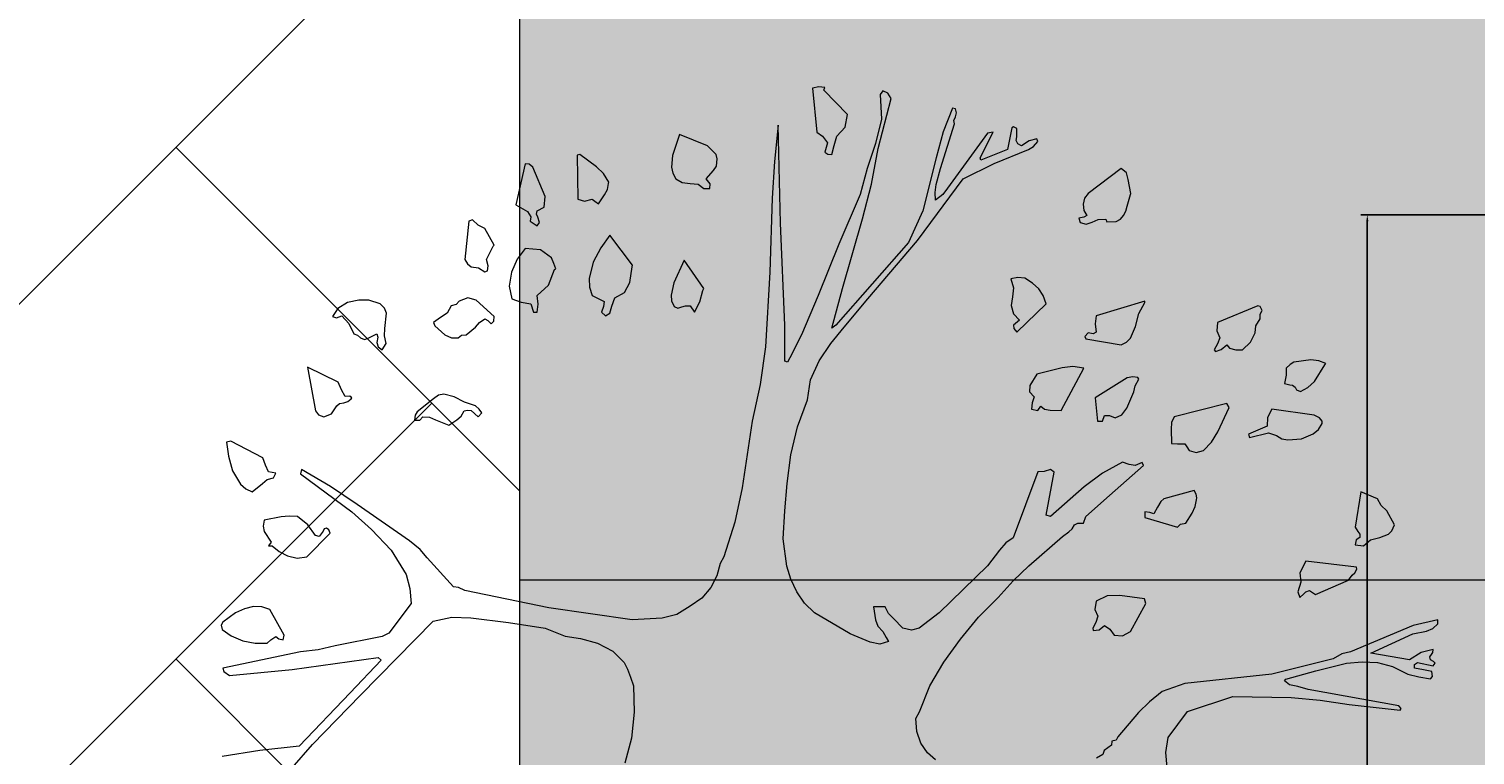
# Model space of a CAD drawing. Units: inches. Extents: x 84 to 1044, y -280 to 906.
# Tile 10 of 105: x 441 to 482, y -46 to -25. Entities that reach past the tile are written whole.
import ezdxf

# ---------------------------------------------------------------- set-up
doc = ezdxf.new("R2010")
doc.units = ezdxf.units.IN
for name, color, linetype, lineweight in [('A-ANNO-DIMS', 2, 'Continuous', 18), ('L-HRDS', 32, 'Continuous', 18), ('L-PLNT', 114, 'Continuous', 15)]:
    doc.layers.add(name, color=color, linetype=linetype, lineweight=lineweight)
for name, color, linetype, lineweight, true_color in [('L-HRDS-PATT', 23, 'Continuous', 9, 0xc2877b), ('L-PLNT-PATT', 9, 'Continuous', 9, 0xafd9aa), ('L-PRKG-PATT', 35, 'Continuous', 9, 0x947764)]:
    doc.layers.add(name, color=color, linetype=linetype, lineweight=lineweight, true_color=true_color)
doc.styles.get("Standard").update_dxf_attribs({"font": 'arial.ttf'})
doc.dimstyles.get("Standard").update_dxf_attribs({"dimtxt": 0.18, "dimasz": 0.18, "dimexe": 0.18, "dimexo": 0.0625, "dimgap": 0.09, "dimtad": 0, "dimtih": 1, "dimtoh": 1, "dimdec": 4, "dimzin": 0, "dimdsep": 46, "dimtxsty": 'Standard', "dimcen": 0.09, "dimadec": 0, "dimazin": 0, "dimtfac": 1, "dimtdec": 4, "dimtofl": 0, "dimtmove": 0, "dimatfit": 3, "dimfxl": 1, "dimtolj": 1, "dimtzin": 0, "dimarcsym": 0})

# ---------------------------------------------------------------- blocks, each defined once
blk = doc.blocks.new('A$C37E508DF')
for p, q in [((0.6329, 1.5111), (0.6367, 1.5175)), ((0.6367, 1.5175), (0.6423, 1.5201)), ((0.6423, 1.5201), (0.6453, 1.5158)), ((0.6453, 1.5158), (0.644, 1.4879)), ((0.6826, 1.493), (0.7096, 1.5209)), ((0.7083, 1.5239), (0.7152, 1.5244)), ((0.7096, 1.5209), (0.7083, 1.5239)), ((0.7152, 1.5244), (0.7225, 1.5231)), ((0.7225, 1.5231), (0.7174, 1.4729)), ((0.5583, 1.4948), (0.5596, 1.4995)), ((0.5596, 1.4995), (0.563, 1.5003)), ((0.563, 1.5003), (0.5737, 1.4733)), ((0.6475, 1.4545), (0.6329, 1.5111)), ((0.5596, 1.4905), (0.5583, 1.4948)), ((0.5613, 1.4862), (0.5596, 1.4905)), ((0.5608, 1.4823), (0.5613, 1.4862)), ((0.644, 1.4879), (0.6505, 1.46)), ((0.6852, 1.4785), (0.6826, 1.493)), ((0.4897, 1.4772), (0.4935, 1.4789)), ((0.4897, 1.4678), (0.4897, 1.4772)), ((0.4905, 1.4635), (0.4897, 1.4678)), ((0.4935, 1.4789), (0.4952, 1.478)), ((0.4952, 1.478), (0.5004, 1.4532)), ((0.5313, 1.4437), (0.5167, 1.4729)), ((0.5167, 1.4729), (0.5231, 1.4716)), ((0.5231, 1.4716), (0.5686, 1.409)), ((0.5767, 1.4317), (0.5608, 1.4823)), ((0.5737, 1.4733), (0.5814, 1.4437)), ((0.6946, 1.4682), (0.6852, 1.4785)), ((0.6976, 1.4579), (0.6946, 1.4682)), ((0.7109, 1.4682), (0.7053, 1.4609)), ((0.7174, 1.4729), (0.7109, 1.4682)), ((0.7589, 1.3691), (0.7615, 1.481)), ((0.7615, 1.481), (0.7658, 1.4395)), ((0.8421, 1.4575), (0.8739, 1.4703)), ((0.8739, 1.4703), (0.882, 1.4463)), ((0.4657, 1.4622), (0.4669, 1.4652)), ((0.4708, 1.4566), (0.4657, 1.4622)), ((0.4669, 1.4652), (0.4755, 1.463)), ((0.4764, 1.4532), (0.4708, 1.4566)), ((0.4755, 1.463), (0.4845, 1.4575)), ((0.5154, 1.4373), (0.4764, 1.4532)), ((0.4845, 1.4575), (0.4884, 1.4596)), ((0.4884, 1.4596), (0.4905, 1.4635)), ((0.5004, 1.4532), (0.5308, 1.4412)), ((0.6552, 1.4137), (0.6475, 1.4545)), ((0.6505, 1.46), (0.6603, 1.4317)), ((0.7002, 1.4476), (0.6976, 1.4579)), ((0.7083, 1.4502), (0.7049, 1.448)), ((0.7053, 1.4609), (0.7083, 1.4502)), ((0.8323, 1.4476), (0.8357, 1.451)), ((0.8357, 1.451), (0.8421, 1.4575)), ((0.551, 1.4197), (0.5154, 1.4373)), ((0.5308, 1.4412), (0.5313, 1.4437)), ((0.5814, 1.4437), (0.5969, 1.3833)), ((0.7049, 1.448), (0.7002, 1.4476)), ((0.7658, 1.4395), (0.7684, 1.3979)), ((0.831, 1.4424), (0.8323, 1.4476)), ((0.8318, 1.4343), (0.831, 1.4424)), ((0.8353, 1.4292), (0.8318, 1.4343)), ((0.8829, 1.433), (0.8816, 1.4262)), ((0.882, 1.4463), (0.8829, 1.433)), ((0.9605, 1.4257), (0.9686, 1.4334)), ((0.9686, 1.4334), (0.9875, 1.4476)), ((0.9875, 1.4476), (0.9905, 1.4467)), ((0.9905, 1.4467), (0.9896, 1.3966)), ((1.0269, 1.3996), (1.0411, 1.433)), ((1.0411, 1.433), (1.045, 1.4365)), ((1.045, 1.4365), (1.0497, 1.4369)), ((1.0497, 1.4369), (1.0604, 1.3901)), ((0.3598, 1.403), (0.3628, 1.4189)), ((0.3628, 1.4189), (0.3649, 1.4266)), ((0.3649, 1.4266), (0.3709, 1.4317)), ((0.3709, 1.4317), (0.4086, 1.403)), ((0.6029, 1.3494), (0.551, 1.4197)), ((0.5814, 1.4133), (0.5767, 1.4317)), ((0.6603, 1.4317), (0.668, 1.4021)), ((0.8434, 1.4197), (0.8353, 1.4292)), ((0.8391, 1.4141), (0.8434, 1.4197)), ((0.8781, 1.4197), (0.8709, 1.4154)), ((0.8816, 1.4262), (0.8781, 1.4197)), ((0.9545, 1.4159), (0.9605, 1.4257)), ((0.3602, 1.4021), (0.3598, 1.403)), ((0.364, 1.3888), (0.3602, 1.4021)), ((0.4086, 1.403), (0.4125, 1.3979)), ((0.5686, 1.409), (0.5741, 1.4021)), ((0.5741, 1.4021), (0.5823, 1.3953)), ((0.5827, 1.4043), (0.5814, 1.4133)), ((0.5823, 1.3953), (0.5827, 1.4043)), ((0.6655, 1.3743), (0.6552, 1.4137)), ((0.668, 1.4021), (0.6925, 1.3455)), ((0.8395, 1.4086), (0.8391, 1.4141)), ((0.846, 1.4086), (0.8395, 1.4086)), ((0.8528, 1.4137), (0.846, 1.4086)), ((0.8619, 1.4146), (0.8528, 1.4137)), ((0.8709, 1.4154), (0.8619, 1.4146)), ((0.9549, 1.4146), (0.9545, 1.4159)), ((0.9558, 1.4077), (0.9549, 1.4146)), ((0.9592, 1.4017), (0.9558, 1.4077)), ((0.966, 1.3914), (0.9592, 1.4017)), ((0.3657, 1.3828), (0.364, 1.3888)), ((0.4134, 1.3837), (0.4099, 1.3781)), ((0.4125, 1.3979), (0.4142, 1.391)), ((0.4142, 1.391), (0.4134, 1.3837)), ((0.7684, 1.3979), (0.771, 1.3134)), ((0.9703, 1.3944), (0.966, 1.3914)), ((0.9733, 1.3966), (0.9703, 1.3944)), ((0.9819, 1.3944), (0.9733, 1.3966)), ((0.9896, 1.3966), (0.9819, 1.3944)), ((1.0282, 1.3876), (1.0269, 1.3996)), ((1.0359, 1.3833), (1.0282, 1.3876)), ((1.0604, 1.3901), (1.0471, 1.3824)), ((0.3683, 1.3781), (0.3657, 1.3828)), ((0.3718, 1.3738), (0.3683, 1.3781)), ((0.3765, 1.3713), (0.3718, 1.3738)), ((0.3872, 1.3708), (0.3765, 1.3713)), ((0.3885, 1.3738), (0.3872, 1.3708)), ((0.3971, 1.3734), (0.3885, 1.3738)), ((0.4039, 1.3704), (0.3971, 1.3734)), ((0.4108, 1.3683), (0.4039, 1.3704)), ((0.4099, 1.3781), (0.4134, 1.376)), ((0.4176, 1.37), (0.4108, 1.3683)), ((0.4134, 1.376), (0.4189, 1.3751)), ((0.4189, 1.3751), (0.4176, 1.37)), ((0.5969, 1.3833), (0.6132, 1.3472)), ((0.6882, 1.2949), (0.6655, 1.3743)), ((0.7538, 1.2529), (0.7589, 1.3691)), ((1.0334, 1.37), (1.0351, 1.376)), ((1.0359, 1.3661), (1.0334, 1.37)), ((1.0351, 1.376), (1.0368, 1.3794)), ((1.0368, 1.3794), (1.0359, 1.3833)), ((1.0441, 1.3717), (1.0359, 1.3661)), ((1.0471, 1.3824), (1.0432, 1.3764)), ((1.0432, 1.3764), (1.0441, 1.3717)), ((1.1033, 1.367), (1.1097, 1.373)), ((1.1097, 1.373), (1.114, 1.3717)), ((1.114, 1.3717), (1.1183, 1.328)), ((0.9274, 1.3215), (0.9532, 1.3554)), ((0.9532, 1.3554), (0.9635, 1.3413)), ((1.0848, 1.3443), (1.0955, 1.3631)), ((1.0955, 1.3631), (1.1033, 1.367)), ((0.6595, 1.2829), (0.6029, 1.3494)), ((0.6132, 1.3472), (0.6959, 1.2529)), ((0.6925, 1.3455), (0.7161, 1.2868)), ((0.9635, 1.3413), (0.9721, 1.325)), ((1.0197, 1.3297), (1.0321, 1.3387)), ((1.0321, 1.3387), (1.0497, 1.3404)), ((1.0497, 1.3404), (1.0587, 1.3284)), ((1.0861, 1.343), (1.0848, 1.3443)), ((1.0938, 1.328), (1.0861, 1.343)), ((0.846, 1.2949), (0.8687, 1.3271)), ((0.8687, 1.3271), (0.8803, 1.3014)), ((0.9279, 1.3194), (0.9274, 1.3215)), ((0.9305, 1.3018), (0.9279, 1.3194)), ((0.9721, 1.325), (0.9768, 1.3061)), ((1.0149, 1.3172), (1.0171, 1.3232)), ((1.0171, 1.3232), (1.0197, 1.3297)), ((1.0587, 1.3284), (1.0651, 1.3134)), ((1.0917, 1.3207), (1.0938, 1.328)), ((1.0925, 1.3151), (1.0917, 1.3207)), ((1.1028, 1.3185), (1.0955, 1.3138)), ((1.111, 1.3194), (1.1028, 1.3185)), ((1.1153, 1.3228), (1.111, 1.3194)), ((1.1183, 1.328), (1.1153, 1.3228)), ((0.4717, 1.3009), (0.4807, 1.3065)), ((0.4807, 1.3065), (0.4884, 1.3074)), ((0.4884, 1.3074), (0.4965, 1.3057)), ((0.4965, 1.3057), (0.4935, 1.2954)), ((0.771, 1.3134), (0.7761, 1.2285)), ((0.8803, 1.3014), (0.8833, 1.2872)), ((0.9365, 1.2902), (0.9305, 1.3018)), ((0.9768, 1.3061), (0.9763, 1.2962)), ((1.0162, 1.3164), (1.0149, 1.3172)), ((1.0231, 1.2988), (1.0162, 1.3164)), ((1.0651, 1.3134), (1.0677, 1.2975)), ((1.0955, 1.3138), (1.0925, 1.3151)), ((0.4562, 1.2774), (0.4597, 1.2868)), ((0.4597, 1.2868), (0.4648, 1.2945)), ((0.4648, 1.2945), (0.4717, 1.3009)), ((0.4935, 1.2954), (0.4948, 1.2855)), ((0.4948, 1.2855), (0.4961, 1.2756)), ((0.7002, 1.2495), (0.6882, 1.2949)), ((0.7161, 1.2868), (0.7349, 1.2422)), ((0.8473, 1.2924), (0.846, 1.2949)), ((0.8507, 1.2795), (0.8473, 1.2924)), ((0.8833, 1.2872), (0.8829, 1.2808)), ((0.9476, 1.2842), (0.9365, 1.2902)), ((0.9733, 1.2868), (0.9596, 1.2799)), ((0.9763, 1.2962), (0.9733, 1.2868)), ((1.0359, 1.2868), (1.0231, 1.2988)), ((1.0347, 1.2769), (1.0359, 1.2868)), ((1.0677, 1.2975), (1.0647, 1.2829)), ((0.2101, 1.2696), (0.2127, 1.2744)), ((0.2127, 1.2654), (0.2101, 1.2696)), ((0.2127, 1.2744), (0.2152, 1.2752)), ((0.2152, 1.2752), (0.2611, 1.2559)), ((0.3439, 1.2804), (0.3992, 1.2636)), ((0.3439, 1.2787), (0.3439, 1.2804)), ((0.3507, 1.2662), (0.3439, 1.2787)), ((0.4897, 1.2452), (0.4562, 1.2774)), ((0.4961, 1.2756), (0.4935, 1.2658)), ((0.6865, 1.2508), (0.6595, 1.2829)), ((0.8567, 1.2679), (0.8507, 1.2795)), ((0.8619, 1.2752), (0.8567, 1.2679)), ((0.867, 1.2752), (0.8619, 1.2752)), ((0.8713, 1.2739), (0.867, 1.2752)), ((0.8756, 1.2726), (0.8713, 1.2739)), ((0.8799, 1.2744), (0.8756, 1.2726)), ((0.8829, 1.2808), (0.8799, 1.2744)), ((0.951, 1.2748), (0.9476, 1.2842)), ((0.9532, 1.2666), (0.951, 1.2748)), ((0.9596, 1.2799), (0.9605, 1.2744)), ((0.9605, 1.2744), (0.9626, 1.2679)), ((1.0359, 1.2679), (1.0347, 1.2769)), ((1.0432, 1.2774), (1.0402, 1.2679)), ((1.0544, 1.2791), (1.0432, 1.2774)), ((1.0647, 1.2829), (1.0544, 1.2791)), ((1.0848, 1.2628), (1.1054, 1.2817)), ((1.1054, 1.2817), (1.1148, 1.2842)), ((1.1148, 1.2842), (1.1247, 1.2804)), ((1.1247, 1.2804), (1.1281, 1.2765)), ((1.1281, 1.2765), (1.1341, 1.2752)), ((1.1341, 1.2752), (1.1384, 1.2666)), ((1.2075, 1.2666), (1.21, 1.2726)), ((1.21, 1.2726), (1.2147, 1.2774)), ((1.2147, 1.2774), (1.2276, 1.2817)), ((1.2276, 1.2817), (1.2392, 1.2817)), ((1.2392, 1.2817), (1.2521, 1.2787)), ((1.2521, 1.2787), (1.2632, 1.2722)), ((1.2632, 1.2722), (1.2692, 1.2628)), ((0.2127, 1.2602), (0.2127, 1.2654)), ((0.2174, 1.2521), (0.2127, 1.2602)), ((0.2182, 1.2443), (0.2174, 1.2521)), ((0.2611, 1.2559), (0.262, 1.2465)), ((0.3546, 1.2516), (0.3507, 1.2662)), ((0.3992, 1.2636), (0.4005, 1.2546)), ((0.4005, 1.2546), (0.3992, 1.2452)), ((0.4935, 1.2658), (0.4867, 1.2589)), ((0.4867, 1.2589), (0.4935, 1.2529)), ((0.4935, 1.2529), (0.4931, 1.2491)), ((0.6959, 1.2529), (0.7002, 1.2495)), ((0.7538, 1.2122), (0.7538, 1.2529)), ((0.9583, 1.2636), (0.9532, 1.2666)), ((0.9626, 1.2679), (0.9583, 1.2636)), ((1.0402, 1.2679), (1.0359, 1.2679)), ((1.0852, 1.2576), (1.0848, 1.2628)), ((1.0883, 1.2546), (1.0852, 1.2576)), ((1.0921, 1.2585), (1.0883, 1.2546)), ((1.0955, 1.2602), (1.0921, 1.2585)), ((1.1015, 1.2559), (1.0955, 1.2602)), ((1.1063, 1.2508), (1.1015, 1.2559)), ((1.1384, 1.2666), (1.1461, 1.2619)), ((1.1526, 1.2521), (1.141, 1.2422)), ((1.1461, 1.2619), (1.1539, 1.2559)), ((1.1539, 1.2559), (1.1526, 1.2521)), ((1.2096, 1.2491), (1.2075, 1.2666)), ((1.2503, 1.2551), (1.2448, 1.2431)), ((1.2585, 1.2636), (1.2503, 1.2551)), ((1.2645, 1.2615), (1.2585, 1.2636)), ((1.2692, 1.2628), (1.2645, 1.2615)), ((0.2234, 1.2336), (0.2182, 1.2443)), ((0.262, 1.2465), (0.2586, 1.2388)), ((0.2586, 1.2388), (0.2611, 1.2319)), ((0.3602, 1.2383), (0.3546, 1.2516)), ((0.3649, 1.2336), (0.3602, 1.2383)), ((0.4112, 1.2375), (0.3709, 1.2306)), ((0.3992, 1.2452), (0.4026, 1.2431)), ((0.4026, 1.2431), (0.4086, 1.2443)), ((0.4086, 1.2443), (0.4121, 1.2401)), ((0.4121, 1.2401), (0.4112, 1.2375)), ((0.4931, 1.2491), (0.4897, 1.2452)), ((0.7015, 1.2323), (0.6865, 1.2508)), ((0.7349, 1.2422), (0.7482, 1.216)), ((1.117, 1.2422), (1.1063, 1.2508)), ((1.1221, 1.2418), (1.117, 1.2422)), ((1.126, 1.2388), (1.1221, 1.2418)), ((1.1337, 1.2388), (1.126, 1.2388)), ((1.141, 1.2422), (1.1337, 1.2388)), ((1.2079, 1.2323), (1.21, 1.2409)), ((1.21, 1.2409), (1.2096, 1.2491)), ((1.2186, 1.2431), (1.2173, 1.2392)), ((1.2173, 1.2392), (1.2186, 1.2332)), ((1.2285, 1.2383), (1.2186, 1.2431)), ((1.2328, 1.2366), (1.2285, 1.2383)), ((1.2371, 1.2388), (1.2328, 1.2366)), ((1.2405, 1.2418), (1.2371, 1.2388)), ((1.2448, 1.2431), (1.2405, 1.2418)), ((0.2328, 1.2251), (0.2234, 1.2336)), ((0.2401, 1.2251), (0.2328, 1.2251)), ((0.2474, 1.2268), (0.2401, 1.2251)), ((0.2504, 1.2306), (0.2474, 1.2268)), ((0.2568, 1.2255), (0.2504, 1.2306)), ((0.2633, 1.2229), (0.2568, 1.2255)), ((0.2611, 1.2319), (0.265, 1.2251)), ((0.265, 1.2251), (0.2633, 1.2229)), ((0.3709, 1.2306), (0.3649, 1.2336)), ((0.7148, 1.2126), (0.7015, 1.2323)), ((0.7761, 1.2285), (0.7821, 1.1856)), ((1.2126, 1.2251), (1.2079, 1.2323)), ((1.2169, 1.2285), (1.2126, 1.2251)), ((1.2186, 1.2332), (1.2169, 1.2285)), ((0.1376, 1.2092), (0.1458, 1.2126)), ((0.1389, 1.2079), (0.1376, 1.2092)), ((0.1505, 1.189), (0.1389, 1.2079)), ((0.1458, 1.2126), (0.1548, 1.2135)), ((0.1548, 1.2135), (0.1741, 1.2109)), ((0.1741, 1.2109), (0.1784, 1.2083)), ((0.1784, 1.2083), (0.1831, 1.204)), ((0.1831, 1.204), (0.1831, 1.1959)), ((0.4134, 1.204), (0.4258, 1.2058)), ((0.4391, 1.156), (0.4134, 1.204)), ((0.4258, 1.2058), (0.4382, 1.2045)), ((0.4382, 1.2045), (0.4669, 1.1972)), ((0.7246, 1.1908), (0.7148, 1.2126)), ((0.7482, 1.216), (0.7508, 1.2109)), ((0.7508, 1.2109), (0.7538, 1.2122)), ((1.2628, 1.1882), (1.2975, 1.2053)), ((1.2975, 1.2053), (1.2885, 1.1556)), ((0.1582, 1.1822), (0.1505, 1.189)), ((0.1848, 1.1865), (0.1788, 1.1852)), ((0.1831, 1.1959), (0.1848, 1.1865)), ((0.3507, 1.1916), (0.352, 1.1933)), ((0.355, 1.1839), (0.3507, 1.1916)), ((0.352, 1.1933), (0.3576, 1.1942)), ((0.3576, 1.1942), (0.364, 1.1929)), ((0.364, 1.1929), (0.4005, 1.1702)), ((0.4669, 1.1972), (0.4747, 1.1843)), ((0.7281, 1.168), (0.7246, 1.1908)), ((1.2589, 1.1792), (1.2628, 1.1882)), ((0.1668, 1.1775), (0.1582, 1.1822)), ((0.1711, 1.1792), (0.1668, 1.1775)), ((0.1728, 1.1826), (0.1711, 1.1792)), ((0.1758, 1.1847), (0.1728, 1.1826)), ((0.1788, 1.1852), (0.1758, 1.1847)), ((0.3563, 1.177), (0.355, 1.1839)), ((0.3645, 1.1586), (0.3563, 1.177)), ((0.4005, 1.1702), (0.3979, 1.1436)), ((0.4751, 1.177), (0.47, 1.1714)), ((0.47, 1.1714), (0.4721, 1.1646)), ((0.4747, 1.1843), (0.4751, 1.177)), ((0.7821, 1.1856), (0.7911, 1.1436)), ((1.1187, 1.1655), (1.1307, 1.1714)), ((1.1307, 1.1714), (1.1423, 1.1744)), ((1.1423, 1.1744), (1.1483, 1.1732)), ((1.1483, 1.1732), (1.1539, 1.1693)), ((1.2469, 1.1702), (1.2495, 1.1723)), ((1.2478, 1.1693), (1.2469, 1.1702)), ((1.2495, 1.1723), (1.2546, 1.1719)), ((1.2546, 1.1719), (1.2589, 1.1792)), ((0.1509, 1.1504), (0.1994, 1.1573)), ((0.1994, 1.1573), (0.2041, 1.1479)), ((0.2478, 1.1594), (0.2504, 1.1637)), ((0.2607, 1.1316), (0.2478, 1.1594)), ((0.2504, 1.1637), (0.3104, 1.1487)), ((0.37, 1.1509), (0.3645, 1.1586)), ((0.4519, 1.1564), (0.4391, 1.156)), ((0.458, 1.1573), (0.4519, 1.1564)), ((0.4622, 1.1607), (0.458, 1.1573)), ((0.4657, 1.156), (0.4622, 1.1607)), ((0.473, 1.1573), (0.4657, 1.156)), ((0.4721, 1.1646), (0.473, 1.1573)), ((0.7396, 1.1371), (0.7281, 1.168)), ((1.099, 1.153), (1.102, 1.1573)), ((1.1033, 1.1487), (1.099, 1.153)), ((1.102, 1.1573), (1.1063, 1.1612)), ((1.111, 1.156), (1.1033, 1.1487)), ((1.1063, 1.1612), (1.1187, 1.1655)), ((1.1153, 1.1564), (1.111, 1.156)), ((1.1191, 1.1556), (1.1153, 1.1564)), ((1.1226, 1.1492), (1.1191, 1.1556)), ((1.1539, 1.1693), (1.1727, 1.1543)), ((1.1727, 1.1543), (1.1749, 1.1504)), ((1.2516, 1.1659), (1.2478, 1.1693)), ((1.2563, 1.1646), (1.2516, 1.1659)), ((1.2611, 1.1637), (1.2563, 1.1646)), ((1.2641, 1.1612), (1.2611, 1.1637)), ((1.2701, 1.1522), (1.2641, 1.1612)), ((1.2885, 1.1556), (1.2851, 1.1509)), ((0.1419, 1.1436), (0.1449, 1.1474)), ((0.1419, 1.141), (0.1419, 1.1436)), ((0.1462, 1.1342), (0.1419, 1.141)), ((0.1449, 1.1474), (0.1509, 1.1504)), ((0.2041, 1.1479), (0.2045, 1.138)), ((0.2045, 1.138), (0.226, 1.129)), ((0.3104, 1.1487), (0.3134, 1.1423)), ((0.3134, 1.1423), (0.3139, 1.1346)), ((0.3778, 1.1474), (0.37, 1.1509)), ((0.3842, 1.15), (0.3778, 1.1474)), ((0.3898, 1.15), (0.3842, 1.15)), ((0.3923, 1.1436), (0.3898, 1.15)), ((0.3979, 1.1436), (0.3923, 1.1436)), ((0.7469, 1.1054), (0.7396, 1.1371)), ((0.7911, 1.1436), (0.8027, 1.0677)), ((1.1273, 1.1453), (1.1226, 1.1492)), ((1.1367, 1.1393), (1.1273, 1.1453)), ((1.1517, 1.1453), (1.1367, 1.1393)), ((1.1586, 1.1483), (1.1517, 1.1453)), ((1.1663, 1.1487), (1.1586, 1.1483)), ((1.1697, 1.1449), (1.1663, 1.1487)), ((1.1757, 1.1449), (1.1697, 1.1449)), ((1.1749, 1.1504), (1.1757, 1.1449)), ((1.2791, 1.1487), (1.2701, 1.1522)), ((1.2851, 1.1509), (1.2791, 1.1487)), ((0.1522, 1.1294), (0.1462, 1.1342)), ((0.1655, 1.1234), (0.1522, 1.1294)), ((0.181, 1.1226), (0.1655, 1.1234)), ((0.1878, 1.1234), (0.181, 1.1226)), ((0.1938, 1.1273), (0.1878, 1.1234)), ((0.2032, 1.1303), (0.1938, 1.1273)), ((0.2247, 1.1251), (0.2032, 1.1303)), ((0.226, 1.129), (0.2247, 1.1251)), ((0.268, 1.1196), (0.2607, 1.1316)), ((0.3139, 1.1346), (0.3134, 1.1183)), ((1.3485, 1.102), (1.385, 1.1209)), ((1.385, 1.1209), (1.3897, 1.1196)), ((0.277, 1.1101), (0.268, 1.1196)), ((0.2856, 1.108), (0.277, 1.1101)), ((0.2933, 1.1101), (0.2856, 1.108)), ((0.2959, 1.1144), (0.2933, 1.1101)), ((0.2984, 1.1179), (0.2959, 1.1144)), ((0.3066, 1.1179), (0.2984, 1.1179)), ((0.3134, 1.1183), (0.3066, 1.1179)), ((0.7512, 1.0728), (0.7469, 1.1054)), ((1.3875, 1.1037), (1.3828, 1.087)), ((1.3897, 1.1196), (1.3875, 1.1037)), ((0.3456, 1.093), (0.3469, 1.0964)), ((0.3842, 1.0591), (0.3456, 1.093)), ((0.3469, 1.0964), (0.355, 1.093)), ((0.355, 1.093), (0.3619, 1.0943)), ((0.3619, 1.0943), (0.3692, 1.0968)), ((0.3692, 1.0968), (0.3923, 1.0844)), ((0.4472, 1.0857), (0.4515, 1.0887)), ((0.4515, 1.0887), (0.4584, 1.0865)), ((1.2713, 1.0694), (1.3044, 1.0887)), ((1.3044, 1.0887), (1.3057, 1.0835)), ((1.3421, 1.0861), (1.3455, 1.0934)), ((1.3455, 1.0934), (1.3485, 1.102)), ((0.3923, 1.0844), (0.4129, 1.069)), ((0.4562, 1.0364), (0.4472, 1.0857)), ((0.4584, 1.0865), (0.4657, 1.0861)), ((0.4657, 1.0861), (0.4939, 1.0107)), ((0.7538, 1.0415), (0.7512, 1.0728)), ((1.3057, 1.0835), (1.2469, 1.0402)), ((1.3335, 1.0844), (1.3421, 1.0861)), ((1.3361, 1.0793), (1.3335, 1.0844)), ((1.3434, 1.0771), (1.3361, 1.0793)), ((1.349, 1.0728), (1.3434, 1.0771)), ((1.3605, 1.063), (1.349, 1.0728)), ((1.3738, 1.072), (1.3678, 1.0664)), ((1.3828, 1.087), (1.3738, 1.072)), ((0.0746, 1.0475), (0.0789, 1.0552)), ((0.0789, 1.0552), (0.0978, 1.063)), ((0.0978, 1.063), (0.1042, 1.0231)), ((0.2847, 1.0565), (0.2856, 1.0604)), ((0.2851, 1.054), (0.2847, 1.0565)), ((0.2856, 1.0604), (0.2877, 1.0647)), ((0.2877, 1.0647), (0.3224, 1.0552)), ((0.3224, 1.0552), (0.3255, 1.0522)), ((0.4112, 1.0351), (0.3842, 1.0591)), ((0.4129, 1.069), (0.4515, 1.0351)), ((0.8027, 1.0677), (0.8108, 1.0287)), ((1.2409, 1.0488), (1.2713, 1.0694)), ((1.3678, 1.0664), (1.3605, 1.063)), ((0.0596, 1.0257), (0.0682, 1.0415)), ((0.0682, 1.0415), (0.0746, 1.0475)), ((0.2864, 1.0463), (0.2851, 1.054)), ((0.2899, 1.039), (0.2864, 1.0463)), ((0.2972, 1.0274), (0.2899, 1.039)), ((0.3255, 1.0522), (0.3293, 1.0458)), ((0.3293, 1.0458), (0.3336, 1.0381)), ((0.3336, 1.0381), (0.3383, 1.0398)), ((0.3383, 1.0398), (0.3439, 1.0402)), ((0.3439, 1.0402), (0.3439, 1.0338)), ((0.7559, 1.0098), (0.7538, 1.0415)), ((1.1813, 1.0072), (1.2409, 1.0488)), ((1.2469, 1.0402), (1.2246, 1.0201)), ((0.0626, 1.0188), (0.0596, 1.0257)), ((0.1042, 1.0231), (0.1012, 1.018)), ((0.3032, 1.0265), (0.2972, 1.0274)), ((0.3066, 1.0231), (0.3032, 1.0265)), ((0.3439, 1.0338), (0.3066, 1.0231)), ((0.4138, 1.0274), (0.4112, 1.0351)), ((0.4202, 1.0274), (0.4138, 1.0274)), ((0.4241, 1.0257), (0.4202, 1.0274)), ((0.4267, 1.0209), (0.4241, 1.0257)), ((0.4515, 1.0351), (0.4562, 1.0364)), ((0.8108, 1.0287), (0.8233, 0.9892)), ((1.2731, 1.0197), (1.2761, 1.0218)), ((1.2761, 1.0218), (1.2786, 1.0209)), ((1.2885, 1.0136), (1.2971, 1.0257)), ((1.2971, 1.0257), (1.3091, 1.0351)), ((1.3091, 1.0351), (1.3185, 1.0355)), ((1.3185, 1.0355), (1.3275, 1.0347)), ((1.3275, 1.0347), (1.3468, 1.0308)), ((1.3468, 1.0308), (1.3481, 1.0239)), ((1.3481, 1.0239), (1.3468, 1.018)), ((0.0665, 1.0149), (0.0626, 1.0188)), ((0.0763, 1.0111), (0.0665, 1.0149)), ((0.087, 1.0085), (0.0763, 1.0111)), ((0.0948, 1.0016), (0.087, 1.0085)), ((0.1012, 1.018), (0.099, 1.0149)), ((0.099, 1.0149), (0.099, 1.0111)), ((0.099, 1.0111), (0.1033, 1.0085)), ((0.1033, 1.0085), (0.1042, 1.0029)), ((0.4305, 1.0175), (0.4267, 1.0209)), ((0.4378, 1.0124), (0.4305, 1.0175)), ((0.476, 0.9789), (0.4378, 1.0124)), ((0.4939, 1.0107), (0.5021, 1.0051)), ((0.5021, 1.0051), (0.5094, 0.9969)), ((0.7516, 0.9785), (0.7559, 1.0098)), ((1.1693, 0.9974), (1.1813, 1.0072)), ((1.2246, 1.0201), (1.2023, 0.9969)), ((1.2718, 1.0162), (1.2731, 1.0197)), ((1.2984, 0.9892), (1.2718, 1.0162)), ((1.2786, 1.0209), (1.2799, 1.0184)), ((1.2799, 1.0184), (1.2842, 1.0124)), ((1.2842, 1.0124), (1.2885, 1.0136)), ((1.3468, 1.018), (1.3391, 1.0059)), ((1.3391, 1.0059), (1.3421, 1.0016)), ((0.1042, 1.0029), (0.0948, 1.0016)), ((0.5094, 0.9969), (0.5231, 0.9789)), ((0.8233, 0.9892), (0.8275, 0.9815)), ((1.1612, 0.9879), (1.1693, 0.9974)), ((1.2023, 0.9969), (1.1852, 0.9691)), ((1.3095, 0.9875), (1.2984, 0.9892)), ((1.3202, 0.9901), (1.3095, 0.9875)), ((1.3297, 0.9952), (1.3202, 0.9901)), ((1.3378, 1.0016), (1.3297, 0.9952)), ((1.3421, 1.0016), (1.3378, 1.0016)), ((0.1025, 0.9751), (0.1029, 0.9772)), ((0.1046, 0.9708), (0.1025, 0.9751)), ((0.1029, 0.9772), (0.1604, 0.9841)), ((0.1604, 0.9841), (0.1672, 0.9708)), ((0.4939, 0.9618), (0.476, 0.9789)), ((0.5231, 0.9789), (0.578, 0.9253)), ((0.7469, 0.9635), (0.7516, 0.9785)), ((0.8275, 0.9815), (0.8314, 0.9673)), ((1.1311, 0.9549), (1.1612, 0.9879)), ((0.1076, 0.9682), (0.1046, 0.9708)), ((0.1119, 0.9626), (0.1076, 0.9682)), ((0.1496, 0.9463), (0.1119, 0.9626)), ((0.1672, 0.9708), (0.1664, 0.9601)), ((0.1664, 0.9601), (0.1698, 0.9493)), ((0.5111, 0.9429), (0.4939, 0.9618)), ((0.7401, 0.9493), (0.7469, 0.9635)), ((0.8314, 0.9673), (0.8383, 0.954)), ((1.1852, 0.9691), (1.1809, 0.9532)), ((0.1565, 0.9506), (0.1496, 0.9463)), ((0.1604, 0.9493), (0.1565, 0.9506)), ((0.1629, 0.9468), (0.1604, 0.9493)), ((0.1672, 0.9429), (0.1629, 0.9468)), ((0.1698, 0.9493), (0.1672, 0.9429)), ((0.3426, 0.936), (0.3443, 0.9412)), ((0.3443, 0.9412), (0.3722, 0.9451)), ((0.3722, 0.9451), (0.3868, 0.9446)), ((0.3868, 0.9446), (0.3992, 0.9386)), ((0.5334, 0.9202), (0.5111, 0.9429)), ((0.7315, 0.9365), (0.7401, 0.9493)), ((0.8383, 0.954), (0.8486, 0.942)), ((0.8486, 0.942), (0.8619, 0.933)), ((1.0227, 0.9309), (1.1183, 0.9506)), ((1.1183, 0.9506), (1.1256, 0.954)), ((1.1256, 0.954), (1.1311, 0.9549)), ((1.1809, 0.9532), (1.1796, 0.936)), ((0.3602, 0.9039), (0.3426, 0.936)), ((0.4009, 0.9292), (0.3975, 0.9215)), ((0.3992, 0.9386), (0.4009, 0.9292)), ((0.578, 0.9253), (0.6011, 0.9077)), ((0.6303, 0.9189), (0.6359, 0.9245)), ((0.6359, 0.9245), (0.6397, 0.9322)), ((0.6397, 0.9322), (0.653, 0.9322)), ((0.653, 0.9322), (0.6505, 0.9172)), ((0.6796, 0.9013), (0.7203, 0.9253)), ((0.7203, 0.9253), (0.7315, 0.9365)), ((0.8619, 0.933), (0.8769, 0.9236)), ((0.8769, 0.9236), (0.8936, 0.9193)), ((0.9279, 0.9172), (1.0227, 0.9309)), ((1.1796, 0.936), (1.2049, 0.9022)), ((1.3241, 0.9), (1.3404, 0.9292)), ((1.3404, 0.9292), (1.3494, 0.9322)), ((1.3494, 0.9322), (1.3592, 0.9326)), ((1.3592, 0.9326), (1.3695, 0.93)), ((1.3695, 0.93), (1.3794, 0.9253)), ((1.3794, 0.9253), (1.394, 0.9146)), ((0.0103, 0.9129), (0.0103, 0.9172)), ((0.0103, 0.9172), (0.0382, 0.9107)), ((0.0159, 0.9073), (0.0103, 0.9129)), ((0.0232, 0.9043), (0.0159, 0.9073)), ((0.0382, 0.9107), (0.1098, 0.8807)), ((0.3838, 0.9069), (0.379, 0.9)), ((0.3898, 0.9107), (0.3838, 0.9069)), ((0.3958, 0.906), (0.3898, 0.9107)), ((0.4026, 0.9052), (0.3958, 0.906)), ((0.3975, 0.9215), (0.3996, 0.9142)), ((0.3996, 0.9142), (0.4031, 0.9077)), ((0.4031, 0.9077), (0.4026, 0.9052)), ((0.554, 0.8953), (0.5334, 0.9202)), ((0.6011, 0.9077), (0.6097, 0.9056)), ((0.6097, 0.9056), (0.6196, 0.9077)), ((0.6196, 0.9077), (0.6303, 0.9189)), ((0.6479, 0.9103), (0.6423, 0.9039)), ((0.6505, 0.9172), (0.6479, 0.9103)), ((0.8936, 0.9193), (0.9279, 0.9172)), ((1.0269, 0.9077), (1.0042, 0.8987)), ((1.0685, 0.9142), (1.0269, 0.9077)), ((1.1114, 0.9198), (1.0685, 0.9142)), ((1.1333, 0.9202), (1.1114, 0.9198)), ((1.1543, 0.9159), (1.1333, 0.9202)), ((1.2371, 0.8314), (1.1543, 0.9159)), ((1.3948, 0.9065), (1.3846, 0.8992)), ((1.394, 0.9146), (1.3957, 0.9112)), ((1.3957, 0.9112), (1.3948, 0.9065)), ((0.0386, 0.9013), (0.0232, 0.9043)), ((0.0866, 0.8794), (0.0386, 0.9013)), ((0.3692, 0.8992), (0.3602, 0.9039)), ((0.379, 0.9), (0.3692, 0.8992)), ((0.5728, 0.8691), (0.554, 0.8953)), ((0.6384, 0.8974), (0.6359, 0.8927)), ((0.6359, 0.8927), (0.6457, 0.8897)), ((0.6423, 0.9039), (0.6384, 0.8974)), ((0.6457, 0.8897), (0.6569, 0.8919)), ((0.6569, 0.8919), (0.6796, 0.9013)), ((0.9673, 0.8906), (0.9498, 0.8816)), ((0.9866, 0.8962), (0.9673, 0.8906)), ((1.0042, 0.8987), (0.9866, 0.8962)), ((1.2049, 0.9022), (1.2126, 0.8983)), ((1.2126, 0.8983), (1.2662, 0.8876)), ((1.3254, 0.8944), (1.3241, 0.9)), ((1.3301, 0.8957), (1.3254, 0.8944)), ((1.3335, 0.8983), (1.3301, 0.8957)), ((1.3395, 0.8944), (1.3335, 0.8983)), ((1.3434, 0.8906), (1.3395, 0.8944)), ((1.3571, 0.8906), (1.3434, 0.8906)), ((1.3713, 0.8936), (1.3571, 0.8906)), ((1.3846, 0.8992), (1.3713, 0.8936)), ((0.0159, 0.8803), (0.0154, 0.8837)), ((0.0154, 0.8837), (0.0292, 0.8803)), ((0.0176, 0.8777), (0.0159, 0.8803)), ((0.0193, 0.8752), (0.0176, 0.8777)), ((0.0184, 0.8717), (0.0193, 0.8752)), ((0.0292, 0.8803), (0.0424, 0.8717)), ((0.0424, 0.8717), (0.0866, 0.8794)), ((0.1098, 0.8807), (0.1196, 0.8786)), ((0.1196, 0.8786), (0.1295, 0.873)), ((0.1295, 0.873), (0.1994, 0.8554)), ((0.9498, 0.8816), (0.9369, 0.8687)), ((1.2169, 0.8743), (1.2135, 0.8713)), ((1.3151, 0.8606), (1.2169, 0.8743)), ((1.2662, 0.8876), (1.2855, 0.8833)), ((1.2855, 0.8833), (1.3057, 0.8807)), ((1.3057, 0.8807), (1.394, 0.8623)), ((0.0133, 0.8679), (0.015, 0.87)), ((0.0154, 0.8649), (0.0133, 0.8679)), ((0.015, 0.87), (0.0184, 0.8717)), ((0.0334, 0.8687), (0.0154, 0.8649)), ((0.0163, 0.8529), (0.0171, 0.8584)), ((0.0171, 0.8584), (0.0266, 0.8602)), ((0.0266, 0.8602), (0.0369, 0.8623)), ((0.0369, 0.8666), (0.0334, 0.8687)), ((0.0369, 0.8623), (0.0369, 0.8666)), ((0.0617, 0.864), (0.0442, 0.8554)), ((0.0789, 0.8687), (0.0617, 0.864)), ((0.0965, 0.8696), (0.0789, 0.8687)), ((0.1141, 0.8679), (0.0965, 0.8696)), ((0.1492, 0.8593), (0.1141, 0.8679)), ((0.1835, 0.8499), (0.1492, 0.8593)), ((0.5887, 0.8421), (0.5728, 0.8691)), ((0.933, 0.861), (0.9296, 0.852)), ((0.9369, 0.8687), (0.933, 0.861)), ((1.2135, 0.8713), (1.2491, 0.834)), ((1.3863, 0.8541), (1.3151, 0.8606)), ((1.3927, 0.8584), (1.3863, 0.8541)), ((1.394, 0.8623), (1.3927, 0.8584)), ((0.0184, 0.8503), (0.0163, 0.8529)), ((0.0317, 0.8524), (0.0184, 0.8503)), ((0.0442, 0.8554), (0.0317, 0.8524)), ((0.1578, 0.8378), (0.1698, 0.8413)), ((0.1698, 0.8413), (0.1792, 0.8434)), ((0.1792, 0.8434), (0.1848, 0.8477)), ((0.1848, 0.8477), (0.1835, 0.8499)), ((0.1994, 0.8554), (0.2984, 0.8447)), ((0.2984, 0.8447), (0.3242, 0.8357)), ((0.6007, 0.8125), (0.5887, 0.8421)), ((0.9262, 0.8421), (0.9257, 0.8121)), ((0.9296, 0.852), (0.9262, 0.8421)), ((0.0545, 0.8194), (0.1578, 0.8378)), ((0.1441, 0.8258), (0.1111, 0.8207)), ((0.1771, 0.8288), (0.1441, 0.8258)), ((0.2436, 0.8301), (0.1771, 0.8288)), ((0.2954, 0.813), (0.2436, 0.8301)), ((0.3242, 0.8357), (0.3387, 0.8241)), ((0.3387, 0.8241), (0.3512, 0.8117)), ((1.2919, 0.7752), (1.2371, 0.8314)), ((1.2491, 0.834), (1.3069, 0.7735)), ((0.0519, 0.8164), (0.0545, 0.8194)), ((0.0532, 0.8143), (0.0519, 0.8164)), ((0.1111, 0.8207), (0.0532, 0.8143)), ((0.3173, 0.7834), (0.2954, 0.813)), ((0.3512, 0.8117), (0.3748, 0.7842)), ((0.6046, 0.8048), (0.6007, 0.8125)), ((0.9257, 0.8121), (0.9287, 0.7825)), ((0.6037, 0.7903), (0.6046, 0.8048)), ((0.3199, 0.7662), (0.3173, 0.7834)), ((0.3748, 0.7842), (0.3765, 0.7804)), ((0.3765, 0.7804), (0.3816, 0.7791)), ((0.3816, 0.7791), (0.382, 0.7744)), ((0.382, 0.7744), (0.3859, 0.7714)), ((0.5913, 0.7658), (0.599, 0.777)), ((0.599, 0.777), (0.6037, 0.7903)), ((0.9287, 0.7825), (0.936, 0.7542)), ((1.3151, 0.7487), (1.2919, 0.7752)), ((0.3186, 0.7491), (0.3199, 0.7662)), ((0.3859, 0.7714), (0.3902, 0.7684)), ((0.3902, 0.7684), (0.3919, 0.7641)), ((0.3919, 0.7641), (0.3988, 0.7598)), ((0.5823, 0.7577), (0.5913, 0.7658)), ((1.3069, 0.7735), (1.352, 0.7684)), ((1.352, 0.7684), (1.3948, 0.7615))]:
    blk.add_line(p, q)
blk = doc.blocks.new('*D28')
at = {"layer": 'A-ANNO-DIMS', "color": 0, "lineweight": -2, "transparency": 16777216}
for p, q in [((484.443, -30.627), (478.69, -30.627)), ((478.87, -30.807), (478.87, -49.227)), ((478.87, -68.013), (478.87, -49.593)), ((484.443, -68.193), (478.69, -68.193))]:
    blk.add_line(p, q, dxfattribs=at)
at = {"layer": 'A-ANNO-DIMS', "color": 0, "transparency": 16777216}
for points in [[(478.84, -30.807), (478.9, -30.807), (478.87, -30.627)], [(478.84, -68.013), (478.9, -68.013), (478.87, -68.193)]]:
    blk.add_solid(points, dxfattribs=at)
at = {"layer": 'Defpoints', "color": 0, "transparency": 16777216}
for p in [(478.87, -30.627), (484.505, -30.627), (484.505, -68.193)]:
    blk.add_point(p, dxfattribs=at)
at = {"layer": 'A-ANNO-DIMS', "color": 0, "transparency": 16777216, "insert": (478.87, -49.41), "char_height": 0.18, "attachment_point": 5}
blk.add_mtext('\\A1;SHRUB 38 TYP.', dxfattribs=at)

msp = doc.modelspace()

# ---------------------------------------------------------------- hatches: boundary and pattern name
at = {"layer": 'L-HRDS-PATT', "transparency": 33554567}
h = msp.add_hatch(color=256, dxfattribs=at)
h.dxf.hatch_style = 1
h.paths.add_polyline_path([(504.574, 31.12), (455.074, 31.12), (455.074, -40.88), (504.574, -40.88)])
at = {"layer": 'L-PLNT-PATT', "transparency": 33554597}
h = msp.add_hatch(color=256, dxfattribs=at)
h.dxf.hatch_style = 1
h.paths.add_polyline_path([(504.574, -40.88), (455.074, -40.88), (455.074, -112.88), (504.574, -112.88)])
at = {"layer": 'L-PRKG-PATT', "transparency": 33554567}
h = msp.add_hatch(dxfattribs=at)
h.set_pattern_fill('AR-HBONE', color=256, scale=0.1)
h.paths.add_polyline_path([(455.074, 31.12), (455.074, 91.12), (455.074, 151.12), (413.127, 151.12), (341.127, 151.12), (290.179, 151.12), (227.179, 151.12), (227.179, 127.12), (143.179, 127.12), (143.179, -112.88), (143.179, -117.88), (455.074, -117.88)])

# ---------------------------------------------------------------- linework, layer by layer
at = {"layer": 'L-HRDS'}
for p, q in [((455.074, 31.12), (455.074, -121.88)), ((504.574, -40.88), (455.074, -40.88))]:
    msp.add_line(p, q, dxfattribs=at)

# ---------------------------------------------------------------- block references
at = {"layer": 'L-PLNT', "xscale": -24.64361536662419, "yscale": 24.64361536662419, "zscale": 24.64361536662419}
msp.add_blockref('A$C37E508DF', (481.101, -64.604), dxfattribs=at)

# ---------------------------------------------------------------- dimensions: what is measured, and where the dimension line sits
at = {"layer": 'A-ANNO-DIMS'}
dim = msp.add_linear_dim(base=(478.87, -30.627), p1=(484.505, -68.193), p2=(484.505, -30.627), angle=90, text='SHRUB <> TYP.', dimstyle='Standard', override={"dimdec": 0, "dimlfac": 1, "dimrnd": 0, "dimzin": 0, "dimdsep": 46, "dimlunit": 2}, dxfattribs=at)
dim.commit()
dim.dimension.update_dxf_attribs({"geometry": '*D28', "text_midpoint": (478.87, -49.41)})

doc.saveas('drawing.dxf')
